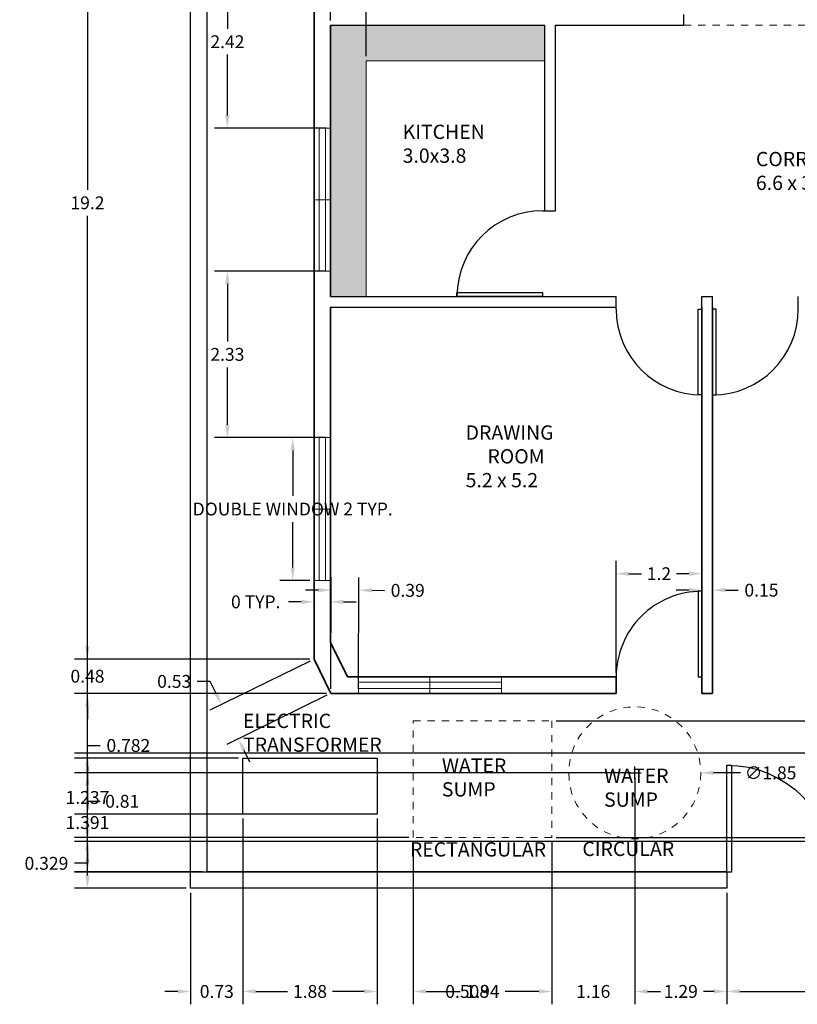
# Model space of a CAD drawing. Units: metres. Extents: x 2527.9 to 2558.5, y 2010.7 to 2033.1.
# Tile 1 of 3: x 2538.2 to 2549.1, y 2010.7 to 2024.5. Entities that reach past the tile are written whole.
import ezdxf

# ---------------------------------------------------------------- set-up
doc = ezdxf.new("R2010")
doc.units = ezdxf.units.M
doc.linetypes.add('ACAD_ISO02W100', pattern=[15, 12, -3])
for name, color, linetype, lineweight in [('A-ANNO-DIMS', 2, 'Continuous', 18), ('A-AREA-IDEN', 180, 'Continuous', 18), ('A-CASE', 8, 'Continuous', 18), ('A-DOOR', 249, 'Continuous', 25), ('A-GLAZ', 249, 'Continuous', 18), ('A-WALL-OVHD', 6, 'ACAD_ISO02W100', 18), ('ANNOTATION', 180, 'Continuous', 18), ('C-SITE-GATE', 249, 'Continuous', 25), ('C-SITE-WALL', 110, 'Continuous', 30), ('E-POWR-EQPM', 7, 'Continuous', 25), ('E-POWR-PATT', 7, 'Continuous', 13), ('INNER WALL', 109, 'Continuous', 30), ('OUTER WALL', 110, 'Continuous', 35), ('P-WATR-TANK', 7, 'ACAD_ISO02W100', 18)]:
    doc.layers.add(name, color=color, linetype=linetype, lineweight=lineweight)
doc.layers.add('A-CASE-PATT', color=251, linetype='Continuous', lineweight=13, true_color=0x636466)
doc.styles.get("Standard").update_dxf_attribs({"font": 'arial.ttf'})
doc.dimstyles.get("Standard").update_dxf_attribs({"dimtxt": 0.18, "dimasz": 0.18, "dimexe": 0.18, "dimexo": 0.0625, "dimgap": 0.09, "dimtad": 0, "dimtih": 1, "dimtoh": 1, "dimdec": 1, "dimzin": 0, "dimdsep": 46, "dimtxsty": 'Standard', "dimcen": 0.09, "dimadec": 0, "dimazin": 0, "dimtfac": 1, "dimtdec": 1, "dimtofl": 0, "dimtmove": 0, "dimatfit": 3, "dimfxl": 1, "dimtolj": 1, "dimtzin": 0, "dimarcsym": 0})

# ---------------------------------------------------------------- blocks, each defined once
blk = doc.blocks.new('*U2')
for p, q in [((0, 0), (0, -6)), ((40, 0), (40, -6))]:
    blk.add_line(p, q)
blk.add_lwpolyline([(0, 0), (0, 40), (1.75, 40), (1.75, 0)], close=True)
blk.add_arc((0, 0), 40, 0, 90)
blk = doc.blocks.new('*U5')
for p, q in [((0, 0), (0, -6)), ((-40, 0), (-40, -6))]:
    blk.add_line(p, q)
blk.add_lwpolyline([(0, 0), (0, 40), (-1.75, 40), (-1.75, 0)], close=True)
blk.add_arc((0, 0), 40, 90, 180)
blk = doc.blocks.new('*U6')
for p, q in [((0, 0), (0, 6)), ((40, 0), (40, 6))]:
    blk.add_line(p, q)
blk.add_lwpolyline([(0, 0), (0, -40), (1.75, -40), (1.75, 0)], close=True)
blk.add_arc((0, 0), 40, 270, 0)
blk = doc.blocks.new('*U7')
for p, q in [((-40, 0), (-40, 6)), ((0, 0), (0, 6))]:
    blk.add_line(p, q)
blk.add_lwpolyline([(0, 0), (0, -40), (-1.75, -40), (-1.75, 0)], close=True)
blk.add_arc((0, 0), 40, 180, 270)
blk = doc.blocks.new('WIN-2000-DOUBLE')
at = {"ltscale": 0.2}
for p, q in [((0, 0.23), (1, 0.23)), ((0, 0), (0, 0.23)), ((0, 0.16), (1, 0.16)), ((1, 0.23), (1, 0)), ((1, 0.23), (2, 0.23)), ((1, 0), (1, 0.23)), ((1, 0.16), (2, 0.16)), ((2, 0.23), (2, 0)), ((1, 0.07), (0, 0.07)), ((1, 0), (0, 0)), ((2, 0.07), (1, 0.07)), ((2, 0), (1, 0))]:
    blk.add_line(p, q, dxfattribs=at)
blk = doc.blocks.new('*D11')
at = {"layer": 'A-ANNO-DIMS', "color": 0, "lineweight": -2, "ltscale": 0.2, "transparency": 16777216}
for p, q in [((2542.221, 2018.626), (2541.803, 2018.626)), ((2541.983, 2018.446), (2541.983, 2017.809)), ((2541.983, 2016.806), (2541.983, 2017.443)), ((2542.221, 2016.626), (2541.803, 2016.626))]:
    blk.add_line(p, q, dxfattribs=at)
at = {"layer": 'A-ANNO-DIMS', "color": 0, "lineweight": -3, "ltscale": 0.2, "transparency": 16777216}
for points in [[(2541.953, 2018.446), (2542.013, 2018.446), (2541.983, 2018.626)], [(2541.953, 2016.806), (2542.013, 2016.806), (2541.983, 2016.626)]]:
    blk.add_solid(points, dxfattribs=at)
at = {"layer": 'Defpoints', "color": 0, "lineweight": -3, "ltscale": 0.2, "transparency": 16777216}
for p in [(2541.983, 2018.626), (2542.283, 2018.626), (2542.283, 2016.626)]:
    blk.add_point(p, dxfattribs=at)
at = {"layer": 'A-ANNO-DIMS', "color": 0, "ltscale": 0.2, "transparency": 16777216, "insert": (2541.983, 2017.626), "char_height": 0.18, "attachment_point": 5}
blk.add_mtext('\\A1;DOUBLE WINDOW 2 TYP.', dxfattribs=at)
blk = doc.blocks.new('*D12')
at = {"layer": 'A-ANNO-DIMS', "color": 0, "lineweight": -2, "ltscale": 0.2, "transparency": 16777216}
for p, q in [((2542.283, 2016.564), (2542.283, 2016.146)), ((2542.513, 2016.564), (2542.513, 2016.146)), ((2542.103, 2016.326), (2541.923, 2016.326)), ((2542.693, 2016.326), (2542.873, 2016.326))]:
    blk.add_line(p, q, dxfattribs=at)
at = {"layer": 'A-ANNO-DIMS', "color": 0, "lineweight": -3, "ltscale": 0.2, "transparency": 16777216}
for points in [[(2542.103, 2016.356), (2542.103, 2016.296), (2542.283, 2016.326)], [(2542.693, 2016.356), (2542.693, 2016.296), (2542.513, 2016.326)]]:
    blk.add_solid(points, dxfattribs=at)
at = {"layer": 'Defpoints', "color": 0, "lineweight": -3, "ltscale": 0.2, "transparency": 16777216}
for p in [(2542.283, 2016.626), (2542.513, 2016.626), (2542.283, 2016.326)]:
    blk.add_point(p, dxfattribs=at)
at = {"layer": 'A-ANNO-DIMS', "color": 0, "ltscale": 0.2, "transparency": 16777216, "insert": (2541.465, 2016.326), "char_height": 0.18, "attachment_point": 5}
blk.add_mtext('\\A1;0 TYP.', dxfattribs=at)
blk = doc.blocks.new('*D18')
at = {"layer": 'A-ANNO-DIMS', "color": 0, "lineweight": -2, "ltscale": 0.2, "transparency": 16777216}
for p, q in [((2540.491, 2031.515), (2538.928, 2031.515)), ((2539.108, 2031.335), (2539.108, 2022.096)), ((2539.108, 2012.495), (2539.108, 2021.733)), ((2540.491, 2012.315), (2538.928, 2012.315))]:
    blk.add_line(p, q, dxfattribs=at)
at = {"layer": 'A-ANNO-DIMS', "color": 0, "lineweight": -3, "ltscale": 0.2, "transparency": 16777216}
for points in [[(2539.078, 2031.335), (2539.138, 2031.335), (2539.108, 2031.515)], [(2539.078, 2012.495), (2539.138, 2012.495), (2539.108, 2012.315)]]:
    blk.add_solid(points, dxfattribs=at)
at = {"layer": 'Defpoints', "color": 0, "lineweight": -3, "ltscale": 0.2, "transparency": 16777216}
for p in [(2539.108, 2031.515), (2540.553, 2031.515), (2540.553, 2012.315)]:
    blk.add_point(p, dxfattribs=at)
at = {"layer": 'A-ANNO-DIMS', "color": 0, "ltscale": 0.2, "transparency": 16777216, "insert": (2539.108, 2021.915), "char_height": 0.18, "attachment_point": 5}
blk.add_mtext('\\A1;19.2', dxfattribs=at)
blk = doc.blocks.new('*D24')
at = {"layer": 'A-ANNO-DIMS', "color": 0, "lineweight": -2, "ltscale": 0.2, "transparency": 16777216}
for p, q in [((2548.064, 2012.252), (2548.064, 2010.69)), ((2551.064, 2012.252), (2551.064, 2010.69)), ((2548.244, 2010.87), (2549.416, 2010.87)), ((2550.884, 2010.87), (2549.713, 2010.87))]:
    blk.add_line(p, q, dxfattribs=at)
at = {"layer": 'A-ANNO-DIMS', "color": 0, "lineweight": -3, "ltscale": 0.2, "transparency": 16777216}
for points in [[(2548.244, 2010.9), (2548.244, 2010.84), (2548.064, 2010.87)], [(2550.884, 2010.9), (2550.884, 2010.84), (2551.064, 2010.87)]]:
    blk.add_solid(points, dxfattribs=at)
at = {"layer": 'Defpoints', "color": 0, "lineweight": -3, "ltscale": 0.2, "transparency": 16777216}
for p in [(2548.064, 2012.315), (2551.064, 2012.315), (2551.064, 2010.87)]:
    blk.add_point(p, dxfattribs=at)
at = {"layer": 'A-ANNO-DIMS', "color": 0, "ltscale": 0.2, "transparency": 16777216, "insert": (2549.564, 2010.87), "char_height": 0.18, "attachment_point": 5}
blk.add_mtext('\\A1;3', dxfattribs=at)
blk = doc.blocks.new('*D25')
at = {"layer": 'A-ANNO-DIMS', "color": 0, "lineweight": -2, "ltscale": 0.2, "transparency": 16777216}
for p, q in [((2541.286121, 2013.290777), (2541.286121, 2010.689536)), ((2540.553329, 2012.252036), (2540.553329, 2010.689536)), ((2540.373329, 2010.869536), (2540.193329, 2010.869536)), ((2541.466121, 2010.869536), (2541.646121, 2010.869536))]:
    blk.add_line(p, q, dxfattribs=at)
at = {"layer": 'A-ANNO-DIMS', "color": 0, "lineweight": -3, "ltscale": 0.2, "transparency": 16777216}
for points in [[(2540.373329, 2010.899536), (2540.373329, 2010.839536), (2540.553329, 2010.869536)], [(2541.466121, 2010.899536), (2541.466121, 2010.839536), (2541.286121, 2010.869536)]]:
    blk.add_solid(points, dxfattribs=at)
at = {"layer": 'Defpoints', "color": 0, "lineweight": -3, "ltscale": 0.2, "transparency": 16777216}
for p in [(2541.286121, 2013.353277), (2540.553329, 2012.314536), (2541.286121, 2010.869536)]:
    blk.add_point(p, dxfattribs=at)
at = {"layer": 'A-ANNO-DIMS', "color": 0, "ltscale": 0.2, "transparency": 16777216, "insert": (2540.919725, 2010.869536), "char_height": 0.18, "attachment_point": 5}
blk.add_mtext('\\A1;0.73', dxfattribs=at)
blk = doc.blocks.new('*D26')
at = {"layer": 'A-ANNO-DIMS', "color": 0, "lineweight": -2, "ltscale": 0.2, "transparency": 16777216}
for p, q in [((2541.286, 2013.291), (2541.286, 2010.69)), ((2543.164, 2013.291), (2543.164, 2010.69)), ((2541.466, 2010.87), (2541.91, 2010.87)), ((2542.984, 2010.87), (2542.541, 2010.87))]:
    blk.add_line(p, q, dxfattribs=at)
at = {"layer": 'A-ANNO-DIMS', "color": 0, "lineweight": -3, "ltscale": 0.2, "transparency": 16777216}
for points in [[(2541.466, 2010.9), (2541.466, 2010.84), (2541.286, 2010.87)], [(2542.984, 2010.9), (2542.984, 2010.84), (2543.164, 2010.87)]]:
    blk.add_solid(points, dxfattribs=at)
at = {"layer": 'Defpoints', "color": 0, "lineweight": -3, "ltscale": 0.2, "transparency": 16777216}
for p in [(2541.286, 2013.353), (2543.164, 2013.353), (2543.164, 2010.87)]:
    blk.add_point(p, dxfattribs=at)
at = {"layer": 'A-ANNO-DIMS', "color": 0, "ltscale": 0.2, "transparency": 16777216, "insert": (2542.225, 2010.87), "char_height": 0.18, "attachment_point": 5}
blk.add_mtext('\\A1;1.88', dxfattribs=at)
blk = doc.blocks.new('*D27')
at = {"layer": 'A-ANNO-DIMS', "color": 0, "lineweight": -2, "ltscale": 0.2, "transparency": 16777216}
for p, q in [((2543.164, 2013.291), (2543.164, 2010.69)), ((2543.672, 2012.962), (2543.672, 2010.69)), ((2542.984, 2010.87), (2542.804, 2010.87)), ((2543.852, 2010.87), (2544.032, 2010.87))]:
    blk.add_line(p, q, dxfattribs=at)
at = {"layer": 'A-ANNO-DIMS', "color": 0, "lineweight": -3, "ltscale": 0.2, "transparency": 16777216}
for points in [[(2542.984, 2010.9), (2542.984, 2010.84), (2543.164, 2010.87)], [(2543.852, 2010.9), (2543.852, 2010.84), (2543.672, 2010.87)]]:
    blk.add_solid(points, dxfattribs=at)
at = {"layer": 'Defpoints', "color": 0, "lineweight": -3, "ltscale": 0.2, "transparency": 16777216}
for p in [(2543.164, 2013.353), (2543.672, 2013.024), (2543.672, 2010.87)]:
    blk.add_point(p, dxfattribs=at)
at = {"layer": 'A-ANNO-DIMS', "color": 0, "ltscale": 0.2, "transparency": 16777216, "insert": (2544.426, 2010.87), "char_height": 0.18, "attachment_point": 5}
blk.add_mtext('\\A1;0.508', dxfattribs=at)
blk = doc.blocks.new('*D28')
at = {"layer": 'A-ANNO-DIMS', "color": 0, "lineweight": -2, "ltscale": 0.2, "transparency": 16777216}
for p, q in [((2543.672, 2012.962), (2543.672, 2010.69)), ((2545.612, 2012.962), (2545.612, 2010.69)), ((2543.852, 2010.87), (2544.327, 2010.87)), ((2545.432, 2010.87), (2544.957, 2010.87))]:
    blk.add_line(p, q, dxfattribs=at)
at = {"layer": 'A-ANNO-DIMS', "color": 0, "lineweight": -3, "ltscale": 0.2, "transparency": 16777216}
for points in [[(2543.852, 2010.9), (2543.852, 2010.84), (2543.672, 2010.87)], [(2545.432, 2010.9), (2545.432, 2010.84), (2545.612, 2010.87)]]:
    blk.add_solid(points, dxfattribs=at)
at = {"layer": 'Defpoints', "color": 0, "lineweight": -3, "ltscale": 0.2, "transparency": 16777216}
for p in [(2543.672, 2013.024), (2545.612, 2013.024), (2545.612, 2010.87)]:
    blk.add_point(p, dxfattribs=at)
at = {"layer": 'A-ANNO-DIMS', "color": 0, "ltscale": 0.2, "transparency": 16777216, "insert": (2544.642, 2010.87), "char_height": 0.18, "attachment_point": 5}
blk.add_mtext('\\A1;1.94', dxfattribs=at)
blk = doc.blocks.new('*D29')
at = {"layer": 'A-ANNO-DIMS', "color": 0, "lineweight": -2, "ltscale": 0.2, "transparency": 16777216}
for p, q in [((2546.773625, 2013.868138), (2546.773625, 2010.689536)), ((2545.611793, 2012.96183), (2545.611793, 2010.689536)), ((2545.431793, 2010.869536), (2545.251793, 2010.869536)), ((2546.953625, 2010.869536), (2547.133625, 2010.869536))]:
    blk.add_line(p, q, dxfattribs=at)
at = {"layer": 'A-ANNO-DIMS', "color": 0, "lineweight": -3, "ltscale": 0.2, "transparency": 16777216}
for points in [[(2545.431793, 2010.899536), (2545.431793, 2010.839536), (2545.611793, 2010.869536)], [(2546.953625, 2010.899536), (2546.953625, 2010.839536), (2546.773625, 2010.869536)]]:
    blk.add_solid(points, dxfattribs=at)
at = {"layer": 'Defpoints', "color": 0, "lineweight": -3, "ltscale": 0.2, "transparency": 16777216}
for p in [(2546.773625, 2013.930638), (2545.611793, 2013.02433), (2546.773625, 2010.869536)]:
    blk.add_point(p, dxfattribs=at)
at = {"layer": 'A-ANNO-DIMS', "color": 0, "ltscale": 0.2, "transparency": 16777216, "insert": (2546.192709, 2010.869536), "char_height": 0.18, "attachment_point": 5}
blk.add_mtext('\\A1;1.16', dxfattribs=at)
blk = doc.blocks.new('*D30')
at = {"layer": 'A-ANNO-DIMS', "color": 0, "lineweight": -2, "ltscale": 0.2, "transparency": 16777216}
for p, q in [((2546.774, 2013.868), (2546.774, 2010.69)), ((2548.064, 2012.252), (2548.064, 2010.69)), ((2546.954, 2010.87), (2547.104, 2010.87)), ((2547.884, 2010.87), (2547.735, 2010.87))]:
    blk.add_line(p, q, dxfattribs=at)
at = {"layer": 'A-ANNO-DIMS', "color": 0, "lineweight": -3, "ltscale": 0.2, "transparency": 16777216}
for points in [[(2546.954, 2010.9), (2546.954, 2010.84), (2546.774, 2010.87)], [(2547.884, 2010.9), (2547.884, 2010.84), (2548.064, 2010.87)]]:
    blk.add_solid(points, dxfattribs=at)
at = {"layer": 'Defpoints', "color": 0, "lineweight": -3, "ltscale": 0.2, "transparency": 16777216}
for p in [(2546.774, 2013.931), (2548.064, 2012.315), (2548.064, 2010.87)]:
    blk.add_point(p, dxfattribs=at)
at = {"layer": 'A-ANNO-DIMS', "color": 0, "ltscale": 0.2, "transparency": 16777216, "insert": (2547.419, 2010.87), "char_height": 0.18, "attachment_point": 5}
blk.add_mtext('\\A1;1.29', dxfattribs=at)
blk = doc.blocks.new('*D36')
at = {"layer": 'A-ANNO-DIMS', "color": 0, "lineweight": -2, "ltscale": 0.2, "transparency": 16777216}
for p, q in [((2539.108, 2014.135), (2539.108, 2014.315)), ((2539.108, 2014.315), (2539.288, 2014.315)), ((2541.224, 2014.135), (2538.928, 2014.135)), ((2539.108, 2013.533), (2539.108, 2013.955)), ((2541.224, 2013.353), (2538.928, 2013.353))]:
    blk.add_line(p, q, dxfattribs=at)
at = {"layer": 'A-ANNO-DIMS', "color": 0, "lineweight": -3, "ltscale": 0.2, "transparency": 16777216}
for points in [[(2539.078, 2013.955), (2539.138, 2013.955), (2539.108, 2014.135)], [(2539.078, 2013.533), (2539.138, 2013.533), (2539.108, 2013.353)]]:
    blk.add_solid(points, dxfattribs=at)
at = {"layer": 'Defpoints', "color": 0, "lineweight": -3, "ltscale": 0.2, "transparency": 16777216}
for p in [(2539.108, 2014.135), (2541.286, 2014.135), (2541.286, 2013.353)]:
    blk.add_point(p, dxfattribs=at)
at = {"layer": 'A-ANNO-DIMS', "color": 0, "ltscale": 0.2, "transparency": 16777216, "insert": (2539.681, 2014.315), "char_height": 0.18, "attachment_point": 5}
blk.add_mtext('\\A1;0.782', dxfattribs=at)
blk = doc.blocks.new('*D37')
at = {"layer": 'A-ANNO-DIMS', "color": 0, "lineweight": -2, "ltscale": 0.2, "transparency": 16777216}
for p, q in [((2545.674, 2014.659), (2558.378, 2014.659)), ((2558.198, 2014.479), (2558.198, 2014.024)), ((2558.198, 2013.204), (2558.198, 2013.66)), ((2545.674, 2013.024), (2558.378, 2013.024))]:
    blk.add_line(p, q, dxfattribs=at)
at = {"layer": 'A-ANNO-DIMS', "color": 0, "lineweight": -3, "ltscale": 0.2, "transparency": 16777216}
for points in [[(2558.168, 2014.479), (2558.228, 2014.479), (2558.198, 2014.659)], [(2558.168, 2013.204), (2558.228, 2013.204), (2558.198, 2013.024)]]:
    blk.add_solid(points, dxfattribs=at)
at = {"layer": 'Defpoints', "color": 0, "lineweight": -3, "ltscale": 0.2, "transparency": 16777216}
for p in [(2545.612, 2014.659), (2558.198, 2014.659), (2545.612, 2013.024)]:
    blk.add_point(p, dxfattribs=at)
at = {"layer": 'A-ANNO-DIMS', "color": 0, "ltscale": 0.2, "transparency": 16777216, "insert": (2558.198, 2013.842), "char_height": 0.18, "attachment_point": 5}
blk.add_mtext('\\A1;1.635', dxfattribs=at)
blk = doc.blocks.new('*D38')
at = {"layer": 'A-ANNO-DIMS', "color": 0, "lineweight": -2, "ltscale": 0.2, "transparency": 16777216}
for p, q in [((2551.326, 2014.205), (2538.928, 2014.205)), ((2539.108, 2014.025), (2539.108, 2013.768)), ((2539.108, 2013.148), (2539.108, 2013.404)), ((2551.326, 2012.968), (2538.928, 2012.968))]:
    blk.add_line(p, q, dxfattribs=at)
at = {"layer": 'A-ANNO-DIMS', "color": 0, "lineweight": -3, "ltscale": 0.2, "transparency": 16777216}
for points in [[(2539.078, 2014.025), (2539.138, 2014.025), (2539.108, 2014.205)], [(2539.078, 2013.148), (2539.138, 2013.148), (2539.108, 2012.968)]]:
    blk.add_solid(points, dxfattribs=at)
at = {"layer": 'Defpoints', "color": 0, "lineweight": -3, "ltscale": 0.2, "transparency": 16777216}
for p in [(2539.108, 2014.205), (2551.389, 2014.205), (2551.389, 2012.968)]:
    blk.add_point(p, dxfattribs=at)
at = {"layer": 'A-ANNO-DIMS', "color": 0, "ltscale": 0.2, "transparency": 16777216, "insert": (2539.108, 2013.586), "char_height": 0.18, "attachment_point": 5}
blk.add_mtext('\\A1;1.237', dxfattribs=at)
blk = doc.blocks.new('*D39')
at = {"layer": 'A-ANNO-DIMS', "color": 0, "lineweight": -2, "ltscale": 0.2, "transparency": 16777216}
for p, q in [((2539.108, 2013.353), (2539.108, 2013.533)), ((2539.108, 2013.533), (2539.288, 2013.533)), ((2541.224, 2013.353), (2538.928, 2013.353)), ((2539.108, 2012.725), (2539.108, 2013.173)), ((2540.721, 2012.545), (2538.928, 2012.545))]:
    blk.add_line(p, q, dxfattribs=at)
at = {"layer": 'A-ANNO-DIMS', "color": 0, "lineweight": -3, "ltscale": 0.2, "transparency": 16777216}
for points in [[(2539.078, 2013.173), (2539.138, 2013.173), (2539.108, 2013.353)], [(2539.078, 2012.725), (2539.138, 2012.725), (2539.108, 2012.545)]]:
    blk.add_solid(points, dxfattribs=at)
at = {"layer": 'Defpoints', "color": 0, "lineweight": -3, "ltscale": 0.2, "transparency": 16777216}
for p in [(2539.108, 2013.353), (2541.286, 2013.353), (2540.783, 2012.545)]:
    blk.add_point(p, dxfattribs=at)
at = {"layer": 'A-ANNO-DIMS', "color": 0, "ltscale": 0.2, "transparency": 16777216, "insert": (2539.595, 2013.533), "char_height": 0.18, "attachment_point": 5}
blk.add_mtext('\\A1;0.81', dxfattribs=at)
blk = doc.blocks.new('*D40')
at = {"layer": 'A-ANNO-DIMS', "color": 0, "lineweight": -2, "ltscale": 0.2, "transparency": 16777216}
for p, q in [((2539.108, 2013.533), (2539.108, 2013.713)), ((2543.102, 2013.353), (2538.928, 2013.353)), ((2543.61, 2013.024), (2538.928, 2013.024)), ((2539.108, 2012.844), (2539.108, 2012.664)), ((2539.108, 2012.664), (2538.928, 2012.664))]:
    blk.add_line(p, q, dxfattribs=at)
at = {"layer": 'A-ANNO-DIMS', "color": 0, "lineweight": -3, "ltscale": 0.2, "transparency": 16777216}
for points in [[(2539.078, 2013.533), (2539.138, 2013.533), (2539.108, 2013.353)], [(2539.078, 2012.844), (2539.138, 2012.844), (2539.108, 2013.024)]]:
    blk.add_solid(points, dxfattribs=at)
at = {"layer": 'Defpoints', "color": 0, "lineweight": -3, "ltscale": 0.2, "transparency": 16777216}
for p in [(2543.164, 2013.353), (2539.108, 2013.024), (2543.672, 2013.024)]:
    blk.add_point(p, dxfattribs=at)
at = {"layer": 'A-ANNO-DIMS', "color": 0, "ltscale": 0.2, "transparency": 16777216, "insert": (2538.534, 2012.664), "char_height": 0.18, "attachment_point": 5}
blk.add_mtext('\\A1;0.329', dxfattribs=at)
blk = doc.blocks.new('*D41')
at = {"layer": 'A-ANNO-DIMS', "color": 0, "lineweight": -2, "ltscale": 0.2, "transparency": 16777216}
for p, q in [((2546.711, 2013.931), (2538.928, 2013.931)), ((2539.108, 2013.751), (2539.108, 2013.417)), ((2539.108, 2012.72), (2539.108, 2013.053)), ((2548.068, 2012.54), (2538.928, 2012.54))]:
    blk.add_line(p, q, dxfattribs=at)
at = {"layer": 'A-ANNO-DIMS', "color": 0, "lineweight": -3, "ltscale": 0.2, "transparency": 16777216}
for points in [[(2539.078, 2013.751), (2539.138, 2013.751), (2539.108, 2013.931)], [(2539.078, 2012.72), (2539.138, 2012.72), (2539.108, 2012.54)]]:
    blk.add_solid(points, dxfattribs=at)
at = {"layer": 'Defpoints', "color": 0, "lineweight": -3, "ltscale": 0.2, "transparency": 16777216}
for p in [(2546.774, 2013.931), (2539.108, 2012.54), (2548.13, 2012.54)]:
    blk.add_point(p, dxfattribs=at)
at = {"layer": 'A-ANNO-DIMS', "color": 0, "ltscale": 0.2, "transparency": 16777216, "insert": (2539.108, 2013.235), "char_height": 0.18, "attachment_point": 5}
blk.add_mtext('\\A1;1.391', dxfattribs=at)
blk = doc.blocks.new('*D47')
at = {"layer": 'A-ANNO-DIMS', "color": 0, "lineweight": -2, "ltscale": 0.2, "transparency": 16777216}
for p, q in [((2547.713, 2015.107), (2547.713, 2016.67)), ((2547.863, 2015.107), (2547.863, 2016.67)), ((2547.533, 2016.49), (2547.353, 2016.49)), ((2548.043, 2016.49), (2548.223, 2016.49))]:
    blk.add_line(p, q, dxfattribs=at)
at = {"layer": 'A-ANNO-DIMS', "color": 0, "lineweight": -3, "ltscale": 0.2, "transparency": 16777216}
for points in [[(2547.533, 2016.52), (2547.533, 2016.46), (2547.713, 2016.49)], [(2548.043, 2016.52), (2548.043, 2016.46), (2547.863, 2016.49)]]:
    blk.add_solid(points, dxfattribs=at)
at = {"layer": 'Defpoints', "color": 0, "lineweight": -3, "ltscale": 0.2, "transparency": 16777216}
for p in [(2547.863, 2016.49), (2547.713, 2015.045), (2547.863, 2015.045)]:
    blk.add_point(p, dxfattribs=at)
at = {"layer": 'A-ANNO-DIMS', "color": 0, "ltscale": 0.2, "transparency": 16777216, "insert": (2548.548, 2016.49), "char_height": 0.18, "attachment_point": 5}
blk.add_mtext('\\A1;0.15', dxfattribs=at)
blk = doc.blocks.new('*D49')
at = {"layer": 'A-ANNO-DIMS', "color": 0, "lineweight": -2, "ltscale": 0.2, "transparency": 16777216}
for p, q in [((2546.513, 2015.337), (2546.513, 2016.9)), ((2547.713, 2015.337), (2547.713, 2016.9)), ((2546.693, 2016.72), (2546.869, 2016.72)), ((2547.533, 2016.72), (2547.358, 2016.72))]:
    blk.add_line(p, q, dxfattribs=at)
at = {"layer": 'A-ANNO-DIMS', "color": 0, "lineweight": -3, "ltscale": 0.2, "transparency": 16777216}
for points in [[(2546.693, 2016.75), (2546.693, 2016.69), (2546.513, 2016.72)], [(2547.533, 2016.75), (2547.533, 2016.69), (2547.713, 2016.72)]]:
    blk.add_solid(points, dxfattribs=at)
at = {"layer": 'Defpoints', "color": 0, "lineweight": -3, "ltscale": 0.2, "transparency": 16777216}
for p in [(2547.713, 2016.72), (2546.513, 2015.275), (2547.713, 2015.275)]:
    blk.add_point(p, dxfattribs=at)
at = {"layer": 'A-ANNO-DIMS', "color": 0, "ltscale": 0.2, "transparency": 16777216, "insert": (2547.113, 2016.72), "char_height": 0.18, "attachment_point": 5}
blk.add_mtext('\\A1;1.2', dxfattribs=at)
blk = doc.blocks.new('*D58')
at = {"layer": 'A-ANNO-DIMS', "color": 0, "lineweight": -2, "ltscale": 0.2, "transparency": 16777216}
for p, q in [((2542.451, 2025.383), (2540.888, 2025.383)), ((2541.068, 2025.203), (2541.068, 2024.351)), ((2541.068, 2023.139), (2541.068, 2023.991)), ((2542.451, 2022.959), (2540.888, 2022.959))]:
    blk.add_line(p, q, dxfattribs=at)
at = {"layer": 'A-ANNO-DIMS', "color": 0, "lineweight": -3, "ltscale": 0.2, "transparency": 16777216}
for points in [[(2541.038, 2025.203), (2541.098, 2025.203), (2541.068, 2025.383)], [(2541.038, 2023.139), (2541.098, 2023.139), (2541.068, 2022.959)]]:
    blk.add_solid(points, dxfattribs=at)
at = {"layer": 'Defpoints', "color": 0, "lineweight": -3, "ltscale": 0.2, "transparency": 16777216}
for p in [(2541.068, 2025.383), (2542.513, 2025.383), (2542.513, 2022.959)]:
    blk.add_point(p, dxfattribs=at)
at = {"layer": 'A-ANNO-DIMS', "color": 0, "ltscale": 0.2, "transparency": 16777216, "insert": (2541.068, 2024.171), "char_height": 0.18, "attachment_point": 5}
blk.add_mtext('\\A1;2.42', dxfattribs=at)
blk = doc.blocks.new('*D59')
at = {"layer": 'A-ANNO-DIMS', "color": 0, "lineweight": -2, "ltscale": 0.2, "transparency": 16777216}
for p, q in [((2542.451, 2020.959), (2540.888, 2020.959)), ((2541.068, 2020.779), (2541.068, 2019.974)), ((2541.068, 2018.806), (2541.068, 2019.61)), ((2542.451, 2018.626), (2540.888, 2018.626))]:
    blk.add_line(p, q, dxfattribs=at)
at = {"layer": 'A-ANNO-DIMS', "color": 0, "lineweight": -3, "ltscale": 0.2, "transparency": 16777216}
for points in [[(2541.038, 2020.779), (2541.098, 2020.779), (2541.068, 2020.959)], [(2541.038, 2018.806), (2541.098, 2018.806), (2541.068, 2018.626)]]:
    blk.add_solid(points, dxfattribs=at)
at = {"layer": 'Defpoints', "color": 0, "lineweight": -3, "ltscale": 0.2, "transparency": 16777216}
for p in [(2541.068, 2020.959), (2542.513, 2020.959), (2542.513, 2018.626)]:
    blk.add_point(p, dxfattribs=at)
at = {"layer": 'A-ANNO-DIMS', "color": 0, "ltscale": 0.2, "transparency": 16777216, "insert": (2541.068, 2019.792), "char_height": 0.18, "attachment_point": 5}
blk.add_mtext('\\A1;2.33', dxfattribs=at)
blk = doc.blocks.new('*D60')
at = {"layer": 'A-ANNO-DIMS', "color": 0, "lineweight": -2, "ltscale": 0.2, "transparency": 16777216}
for p, q in [((2542.519, 2015.107), (2542.523, 2016.67)), ((2542.906, 2015.106), (2542.911, 2016.668)), ((2542.343, 2016.49), (2542.163, 2016.491)), ((2543.09, 2016.488), (2543.27, 2016.487))]:
    blk.add_line(p, q, dxfattribs=at)
at = {"layer": 'A-ANNO-DIMS', "color": 0, "lineweight": -3, "ltscale": 0.2, "transparency": 16777216}
for points in [[(2542.343, 2016.52), (2542.343, 2016.46), (2542.523, 2016.49)], [(2543.09, 2016.518), (2543.09, 2016.458), (2542.91, 2016.488)]]:
    blk.add_solid(points, dxfattribs=at)
at = {"layer": 'Defpoints', "color": 0, "lineweight": -3, "ltscale": 0.2, "transparency": 16777216}
for p in [(2542.91, 2016.488), (2542.518, 2015.045), (2542.906, 2015.043)]:
    blk.add_point(p, dxfattribs=at)
at = {"layer": 'A-ANNO-DIMS', "color": 0, "ltscale": 0.2, "transparency": 16777216, "insert": (2543.594, 2016.487), "char_height": 0.18, "attachment_point": 5}
blk.add_mtext('\\A1;0.39', dxfattribs=at)
blk = doc.blocks.new('*D61')
at = {"layer": 'A-ANNO-DIMS', "color": 0, "lineweight": -2, "ltscale": 0.2, "transparency": 16777216}
for p, q in [((2539.108329, 2015.704536), (2539.108329, 2015.884536)), ((2542.220829, 2015.524536), (2538.928329, 2015.524536)), ((2542.455824, 2015.044536), (2538.928329, 2015.044536)), ((2539.108329, 2014.864536), (2539.108329, 2014.684536))]:
    blk.add_line(p, q, dxfattribs=at)
at = {"layer": 'A-ANNO-DIMS', "color": 0, "lineweight": -3, "ltscale": 0.2, "transparency": 16777216}
for points in [[(2539.078329, 2015.704536), (2539.138329, 2015.704536), (2539.108329, 2015.524536)], [(2539.078329, 2014.864536), (2539.138329, 2014.864536), (2539.108329, 2015.044536)]]:
    blk.add_solid(points, dxfattribs=at)
at = {"layer": 'Defpoints', "color": 0, "lineweight": -3, "ltscale": 0.2, "transparency": 16777216}
for p in [(2542.283329, 2015.524536), (2539.108329, 2015.044536), (2542.518324, 2015.044536)]:
    blk.add_point(p, dxfattribs=at)
at = {"layer": 'A-ANNO-DIMS', "color": 0, "ltscale": 0.2, "transparency": 16777216, "insert": (2539.108329, 2015.284536), "char_height": 0.18, "attachment_point": 5}
blk.add_mtext('\\A1;0.48', dxfattribs=at)
blk = doc.blocks.new('*D62')
at = {"layer": 'A-ANNO-DIMS', "color": 0, "lineweight": -2, "ltscale": 0.2, "transparency": 16777216}
for p, q in [((2542.227, 2015.497), (2540.824, 2014.81)), ((2540.827, 2015.212), (2540.647, 2015.212)), ((2540.906, 2015.051), (2540.827, 2015.212)), ((2542.462, 2015.017), (2541.059, 2014.33)), ((2541.3, 2014.247), (2541.379, 2014.086))]:
    blk.add_line(p, q, dxfattribs=at)
at = {"layer": 'A-ANNO-DIMS', "color": 0, "lineweight": -3, "ltscale": 0.2, "transparency": 16777216}
for points in [[(2540.933, 2015.064), (2540.879, 2015.038), (2540.986, 2014.889)], [(2541.327, 2014.261), (2541.273, 2014.234), (2541.221, 2014.409)]]:
    blk.add_solid(points, dxfattribs=at)
at = {"layer": 'Defpoints', "color": 0, "lineweight": -3, "ltscale": 0.2, "transparency": 16777216}
for p in [(2542.283, 2015.525), (2542.518, 2015.045), (2540.986, 2014.889)]:
    blk.add_point(p, dxfattribs=at)
at = {"layer": 'A-ANNO-DIMS', "color": 0, "ltscale": 0.2, "transparency": 16777216, "insert": (2540.323, 2015.212), "char_height": 0.18, "attachment_point": 5}
blk.add_mtext('\\A1;0.53', dxfattribs=at)
blk = doc.blocks.new('*D65')
at = {"layer": 'A-ANNO-DIMS', "color": 0, "lineweight": -2, "ltscale": 0.2, "transparency": 16777216}
for p, q in [((2542.513, 2024.467), (2542.513, 2033.14)), ((2543.013, 2023.967), (2543.013, 2033.14)), ((2542.333, 2032.96), (2542.153, 2032.96)), ((2543.193, 2032.96), (2543.373, 2032.96))]:
    blk.add_line(p, q, dxfattribs=at)
at = {"layer": 'A-ANNO-DIMS', "color": 0, "lineweight": -3, "ltscale": 0.2, "transparency": 16777216}
for points in [[(2542.333, 2032.99), (2542.333, 2032.93), (2542.513, 2032.96)], [(2543.193, 2032.99), (2543.193, 2032.93), (2543.013, 2032.96)]]:
    blk.add_solid(points, dxfattribs=at)
at = {"layer": 'Defpoints', "color": 0, "lineweight": -3, "ltscale": 0.2, "transparency": 16777216}
for p in [(2542.513, 2032.96), (2542.513, 2024.405), (2543.013, 2023.905)]:
    blk.add_point(p, dxfattribs=at)
at = {"layer": 'A-ANNO-DIMS', "color": 0, "ltscale": 0.2, "transparency": 16777216, "insert": (2541.899, 2032.96), "char_height": 0.18, "attachment_point": 5}
blk.add_mtext('\\A1;0.5', dxfattribs=at)
blk = doc.blocks.new('*D67')
at = {"layer": 'A-ANNO-DIMS', "color": 0, "lineweight": -2, "ltscale": 0.2, "transparency": 16777216}
for p, q in [((2546.684, 2013.931), (2546.864, 2013.931)), ((2546.774, 2013.841), (2546.774, 2014.021)), ((2548.254, 2013.931), (2547.879, 2013.931))]:
    blk.add_line(p, q, dxfattribs=at)
at = {"layer": 'A-ANNO-DIMS', "color": 0, "lineweight": -3, "ltscale": 0.2, "transparency": 16777216}
blk.add_solid([(2547.879, 2013.961), (2547.879, 2013.901), (2547.699, 2013.931)], dxfattribs=at)
at = {"layer": 'Defpoints', "color": 0, "lineweight": -3, "ltscale": 0.2, "transparency": 16777216}
for p in [(2545.848, 2013.93), (2547.699, 2013.931)]:
    blk.add_point(p, dxfattribs=at)
at = {"layer": 'A-ANNO-DIMS', "color": 0, "ltscale": 0.2, "transparency": 16777216, "insert": (2548.677, 2013.931), "char_height": 0.18, "attachment_point": 5}
blk.add_mtext('\\A1;∅1.85', dxfattribs=at)

msp = doc.modelspace()

# ---------------------------------------------------------------- hatches: boundary and pattern name
at = {"layer": 'A-CASE-PATT', "ltscale": 0.5}
h = msp.add_hatch(color=256, dxfattribs=at)
h.dxf.hatch_style = 1
h.paths.add_polyline_path([(2545.5133, 2024.4045), (2542.5133, 2024.4045), (2542.5133, 2020.6045), (2543.0133, 2020.6045), (2543.0133, 2023.9045), (2545.5133, 2023.9045)])
at = {"layer": 'E-POWR-PATT', "ltscale": 0.005}
h = msp.add_hatch(dxfattribs=at)
h.set_pattern_fill('ACAD_ISO15W100', color=256)
h.set_pattern_definition([(0, (-13.4034, 2e-13), (0, 5), [12, -3, 12, -3, 0.5, -10]), (0, (-13.4034, 2e-13), (0, 5), [-33.5, 0.5, -3, 0.5, -3])])
h.paths.add_polyline_path([(2529.7609, 2014.1352), (2527.8827, 2014.1352), (2527.8827, 2013.3533), (2529.7609, 2013.3533)])
h.paths.add_polyline_path([(2542.889, 2013.9319), (2541.3003, 2013.9319), (2541.3003, 2013.4628), (2542.889, 2013.4628)])
h = msp.add_hatch(dxfattribs=at)
h.set_pattern_fill('ACAD_ISO15W100', color=256)
h.paths.add_polyline_path([(2541.2861, 2014.1352), (2541.2861, 2013.3533), (2543.1643, 2013.3533), (2543.1643, 2014.1352)])
h.paths.add_polyline_path([(2555.5238, 2013.9579), (2553.935, 2013.9579), (2553.935, 2013.4887), (2555.5238, 2013.4887)])

# ---------------------------------------------------------------- linework, layer by layer
at = {"layer": 'A-CASE'}
for p, q in [((2543.0133, 2023.9045), (2545.5133, 2023.9045)), ((2543.0133, 2020.6045), (2543.0133, 2023.9045))]:
    msp.add_line(p, q, dxfattribs=at)
at = {"layer": 'A-WALL-OVHD', "ltscale": 0.002}
msp.add_line((2547.4633, 2024.4045), (2549.9633, 2024.4045), dxfattribs=at)
at = {"layer": 'C-SITE-WALL', "ltscale": 0.5}
msp.add_line((2548.0644, 2012.5445), (2548.0644, 2012.3145), dxfattribs=at)
at = {"layer": 'C-SITE-WALL'}
for points in [[(2548.0644, 2012.3145), (2540.5533, 2012.3145), (2540.5533, 2031.5145)], [(2548.0644, 2012.5445), (2540.7833, 2012.5445), (2540.7833, 2031.2845)]]:
    msp.add_lwpolyline(points, dxfattribs=at)
at = {"layer": 'E-POWR-EQPM', "ltscale": 0.005}
msp.add_lwpolyline([(2541.2861, 2014.1352), (2543.1643, 2014.1352), (2543.1643, 2013.3533), (2541.2861, 2013.3533)], close=True, dxfattribs=at)
at = {"layer": 'INNER WALL'}
for p, q in [((2547.4633, 2024.4045), (2547.4633, 2024.5545)), ((2542.5133, 2024.4045), (2545.5133, 2024.4045)), ((2545.5133, 2021.8045), (2545.5133, 2024.4045)), ((2545.6633, 2021.8045), (2545.6633, 2024.4045)), ((2545.6633, 2024.4045), (2547.4633, 2024.4045)), ((2545.5133, 2021.8045), (2545.6633, 2021.8045)), ((2542.5133, 2020.6045), (2545.5133, 2020.6045)), ((2545.5133, 2020.6045), (2545.6633, 2020.6045)), ((2545.6633, 2020.6045), (2546.5133, 2020.6045)), ((2546.5133, 2020.4545), (2546.5133, 2020.6045)), ((2547.7133, 2020.4545), (2547.7133, 2020.6045)), ((2547.7133, 2020.6045), (2547.8633, 2020.6045)), ((2547.8633, 2020.4545), (2547.8633, 2020.6045)), ((2542.5133, 2020.4545), (2546.5133, 2020.4545))]:
    msp.add_line(p, q, dxfattribs=at)
at = {"layer": 'OUTER WALL'}
for p, q in [((2542.2833, 2015.5245), (2542.2833, 2028.2145)), ((2542.5133, 2020.6045), (2542.5133, 2024.4045)), ((2542.5133, 2015.7545), (2542.5133, 2020.4545)), ((2547.7133, 2015.2745), (2547.7133, 2020.4545)), ((2547.8633, 2015.0445), (2547.8633, 2020.4545)), ((2542.5133, 2015.7545), (2542.7483, 2015.2745)), ((2542.2833, 2015.5245), (2542.5183, 2015.0445)), ((2546.5133, 2015.2745), (2542.7483, 2015.2745)), ((2546.5133, 2015.2745), (2546.5133, 2015.0445)), ((2547.7133, 2015.2745), (2547.7133, 2015.0445)), ((2546.5133, 2015.0445), (2542.5183, 2015.0445)), ((2547.8633, 2015.0445), (2547.7133, 2015.0445))]:
    msp.add_line(p, q, dxfattribs=at)
at = {"layer": 'P-WATR-TANK', "ltscale": 0.005}
msp.add_lwpolyline([(2543.6723, 2014.6594), (2545.6118, 2014.6594), (2545.6118, 2013.0243), (2543.6723, 2013.0243)], close=True, dxfattribs=at)
msp.add_circle((2546.7736, 2013.9306), 0.9253, dxfattribs=at)

# ---------------------------------------------------------------- block references
at = {"layer": 'A-DOOR', "xscale": 0.0299999999999995, "yscale": 0.0299999999999995, "zscale": 0.0299999999999995}
for name, p, rotation in [('*U7', (2545.4833, 2020.6045), 269.9999999999578), ('*U2', (2547.7133, 2020.4245), 179.9999999999577), ('*U5', (2547.8633, 2020.4245), 179.9999999999577), ('*U6', (2547.7133, 2015.2745), 179.9999999999577)]:
    msp.add_blockref(name, p, dxfattribs=dict(at, rotation=rotation))
at = {"layer": 'A-GLAZ'}
for p, rotation in [((2542.5133, 2020.9587), 90.00000000003904), ((2542.5133, 2016.6261), 90.00000000003458)]:
    msp.add_blockref('WIN-2000-DOUBLE', p, dxfattribs=dict(at, rotation=rotation))
msp.add_blockref('WIN-2000-DOUBLE', (2542.9057, 2015.0434), dxfattribs=at)
at = {"layer": 'C-SITE-GATE', "xscale": -0.0374999999999908, "yscale": 0.0374999999999908, "zscale": 0.0374999999999908, "rotation": 180}
msp.add_blockref('*U6', (2548.0644, 2012.5395), dxfattribs=at)

# ---------------------------------------------------------------- texts
at = {"layer": 'A-AREA-IDEN', "char_height": 0.2, "attachment_point": 1}
for s, width, insert in [('KITCHEN   3.0x3.8', 1.274216, (2543.5226, 2023.0087)), ('CORRIDOR-2   6.6 x 3.8', 1.770765, (2548.4709, 2022.6278)), ('DRAWING        ROOM  5.2 x 5.2', 1.373196, (2544.4049, 2018.7974))]:
    msp.add_mtext_dynamic_manual_height_columns(s, width=width, gutter_width=12.5, heights=[0], dxfattribs=dict(at, insert=insert))
at = {"layer": 'ANNOTATION', "char_height": 0.2, "attachment_point": 1}
for s, width, gutter_width, heights, insert in [('ELECTRIC\\PTRANSFORMER\\P', 2.063815, 0.2422, [0.8274], (2541.2861, 2014.7594)), ('WATER SUMP', 1.205045, 12.5, [0.541], (2544.0721, 2014.1336)), ('WATER SUMP', 1.205045, 12.5, [0.541], (2546.3444, 2013.9901)), ('RECTANGULAR', 1.522595, 12.5, [0], (2543.6243, 2012.9592)), ('CIRCULAR', 1.522595, 12.5, [0], (2546.0402, 2012.9666))]:
    msp.add_mtext_dynamic_manual_height_columns(s, width=width, gutter_width=gutter_width, heights=heights, dxfattribs=dict(at, insert=insert))

# ---------------------------------------------------------------- dimensions: what is measured, and where the dimension line sits
at = {"layer": 'A-ANNO-DIMS', "ltscale": 0.2}
for base, p1, p2, override, picture, middle in [((2542.5133, 2032.9595), (2543.0133, 2023.9045), (2542.5133, 2024.4045), {"dimdec": 1, "dimlfac": 1, "dimrnd": 0, "dimzin": 0, "dimdsep": 46, "dimlunit": 2}, '*D65', (2541.8988, 2032.9595)), ((2547.7133, 2016.7195), (2546.5133, 2015.2745), (2547.7133, 2015.2745), {"dimdec": 1, "dimlfac": 1, "dimrnd": 0, "dimzin": 0, "dimdsep": 46, "dimlunit": 2}, '*D49', (2547.1133, 2016.7195)), ((2547.8633, 2016.4895), (2547.7133, 2015.0445), (2547.8633, 2015.0445), {"dimdec": 2, "dimlfac": 1, "dimrnd": 0, "dimzin": 0, "dimdsep": 46, "dimlunit": 2}, '*D47', (2548.5478, 2016.4895)), ((2546.7736, 2010.8695), (2545.6118, 2013.0243), (2546.7736, 2013.9306), {"dimdec": 2, "dimlfac": 1, "dimrnd": 0, "dimzin": 0, "dimdsep": 46, "dimlunit": 2}, '*D29', (2546.1927, 2010.8695)), ((2548.0644, 2010.8695), (2546.7736, 2013.9306), (2548.0644, 2012.3145), {"dimdec": 2, "dimlfac": 1, "dimrnd": 0, "dimzin": 0, "dimdsep": 46, "dimlunit": 2}, '*D30', (2547.419, 2010.8695)), ((2541.2861, 2010.8695), (2540.5533, 2012.3145), (2541.2861, 2013.3533), {"dimdec": 2, "dimlfac": 1, "dimrnd": 0, "dimzin": 0, "dimdsep": 46, "dimlunit": 2}, '*D25', (2540.9197, 2010.8695)), ((2543.1643, 2010.8695), (2541.2861, 2013.3533), (2543.1643, 2013.3533), {"dimdec": 2, "dimlfac": 1, "dimrnd": 0, "dimzin": 0, "dimdsep": 46, "dimlunit": 2}, '*D26', (2542.2252, 2010.8695)), ((2543.6723, 2010.8695), (2543.1643, 2013.3533), (2543.6723, 2013.0243), {"dimdec": 3, "dimlfac": 1, "dimrnd": 0, "dimzin": 0, "dimdsep": 46, "dimlunit": 2}, '*D27', (2544.4262, 2010.8695)), ((2545.6118, 2010.8695), (2543.6723, 2013.0243), (2545.6118, 2013.0243), {"dimdec": 2, "dimlfac": 1, "dimrnd": 0, "dimzin": 0, "dimdsep": 46, "dimlunit": 2}, '*D28', (2544.6421, 2010.8695)), ((2551.0644, 2010.8695), (2548.0644, 2012.3145), (2551.0644, 2012.3145), {"dimdec": 0, "dimlfac": 1, "dimrnd": 0, "dimzin": 0, "dimdsep": 46, "dimlunit": 2}, '*D24', (2549.5644, 2010.8695))]:
    dim = msp.add_linear_dim(base=base, p1=p1, p2=p2, dimstyle='Standard', override=override, dxfattribs=at)
    dim.commit()
    dim.dimension.update_dxf_attribs({"geometry": picture, "text_midpoint": middle})
for base, p1, p2, angle, override, picture, middle in [((2539.1083, 2031.5145), (2540.5533, 2012.3145), (2540.5533, 2031.5145), 90, {"dimdec": 1, "dimlfac": 1, "dimrnd": 0, "dimzin": 0, "dimdsep": 46, "dimlunit": 2}, '*D18', (2539.1083, 2021.9145)), ((2541.0683, 2025.3831), (2542.5133, 2022.9587), (2542.5133, 2025.3831), 90, {"dimdec": 2, "dimlfac": 1, "dimrnd": 0, "dimzin": 0, "dimdsep": 46, "dimlunit": 2}, '*D58', (2541.0683, 2024.1709)), ((2541.0683, 2020.9587), (2542.5133, 2018.6261), (2542.5133, 2020.9587), 90, {"dimdec": 2, "dimlfac": 1, "dimrnd": 0, "dimzin": 0, "dimdsep": 46, "dimlunit": 2}, '*D59', (2541.0683, 2019.7924)), ((2542.9101, 2016.4884), (2542.5183, 2015.0445), (2542.9057, 2015.0434), 359.82806, {"dimdec": 2, "dimlfac": 1, "dimrnd": 0, "dimzin": 0, "dimdsep": 46, "dimlunit": 2}, '*D60', (2543.594, 2016.4873)), ((2539.1083, 2015.0445), (2542.2833, 2015.5245), (2542.5183, 2015.0445), 90, {"dimdec": 2, "dimlfac": 1, "dimrnd": 0, "dimzin": 0, "dimdsep": 46, "dimlunit": 2}, '*D61', (2539.1083, 2015.2845)), ((2540.9855, 2014.8892), (2542.5183, 2015.0445), (2542.2833, 2015.5245), 116.08508, {"dimdec": 2, "dimlfac": 1, "dimrnd": 0, "dimzin": 0, "dimdsep": 46, "dimlunit": 2}, '*D62', (2540.3234, 2015.2125)), ((2558.1983, 2014.6594), (2545.6118, 2013.0243), (2545.6118, 2014.6594), 90, {"dimdec": 3, "dimlfac": 1, "dimrnd": 0, "dimzin": 0, "dimdsep": 46, "dimlunit": 2}, '*D37', (2558.1983, 2013.8419)), ((2539.1083, 2014.1352), (2541.2861, 2013.3533), (2541.2861, 2014.1352), 90, {"dimdec": 3, "dimlfac": 1, "dimrnd": 0, "dimzin": 0, "dimdsep": 46, "dimlunit": 2}, '*D36', (2539.6811, 2014.3152)), ((2539.1083, 2014.2049), (2551.3887, 2012.9678), (2551.3887, 2014.2049), 90, {"dimdec": 3, "dimlfac": 1, "dimrnd": 0, "dimzin": 0, "dimdsep": 46, "dimlunit": 2}, '*D38', (2539.1083, 2013.5863)), ((2539.1083, 2012.5395), (2546.7736, 2013.9306), (2548.1301, 2012.5395), 90, {"dimdec": 3, "dimlfac": 1, "dimrnd": 0, "dimzin": 0, "dimdsep": 46, "dimlunit": 2}, '*D41', (2539.1083, 2013.2351)), ((2539.1083, 2013.0243), (2543.1643, 2013.3533), (2543.6723, 2013.0243), 90, {"dimdec": 3, "dimlfac": 1, "dimrnd": 0, "dimzin": 0, "dimdsep": 46, "dimlunit": 2}, '*D40', (2538.5344, 2012.6643)), ((2539.1083, 2013.3533), (2540.7833, 2012.5445), (2541.2861, 2013.3533), 90, {"dimdec": 2, "dimlfac": 1, "dimrnd": 0, "dimzin": 0, "dimdsep": 46, "dimlunit": 2}, '*D39', (2539.5947, 2013.5333))]:
    dim = msp.add_linear_dim(base=base, p1=p1, p2=p2, angle=angle, dimstyle='Standard', override=override, dxfattribs=at)
    dim.commit()
    dim.dimension.update_dxf_attribs({"geometry": picture, "text_midpoint": middle})
for base, p1, p2, angle, text, picture, middle in [((2541.9833, 2018.6261), (2542.2833, 2016.6261), (2542.2833, 2018.6261), 90, 'DOUBLE WINDOW <> TYP.', '*D11', (2541.9833, 2017.6261)), ((2542.2833, 2016.3261), (2542.5133, 2016.6261), (2542.2833, 2016.6261), 180, '<> TYP.', '*D12', (2541.4652, 2016.3261))]:
    dim = msp.add_linear_dim(base=base, p1=p1, p2=p2, angle=angle, text=text, dimstyle='Standard', override={"dimdec": 0, "dimlfac": 1, "dimrnd": 0, "dimzin": 0, "dimdsep": 46, "dimlunit": 2}, dxfattribs=at)
    dim.commit()
    dim.dimension.update_dxf_attribs({"geometry": picture, "text_midpoint": middle})
dim = msp.add_diameter_dim_2p(p1=(2545.8483, 2013.9303), p2=(2547.6989, 2013.931), dimstyle='Standard', override={"dimdec": 2, "dimlfac": 1, "dimrnd": 0, "dimzin": 0, "dimdsep": 46, "dimlunit": 2}, dxfattribs=at)
dim.commit()
dim.dimension.update_dxf_attribs({"geometry": '*D67', "text_midpoint": (2548.2541, 2013.9312), "dimtype": 163})

doc.saveas('drawing.dxf')
